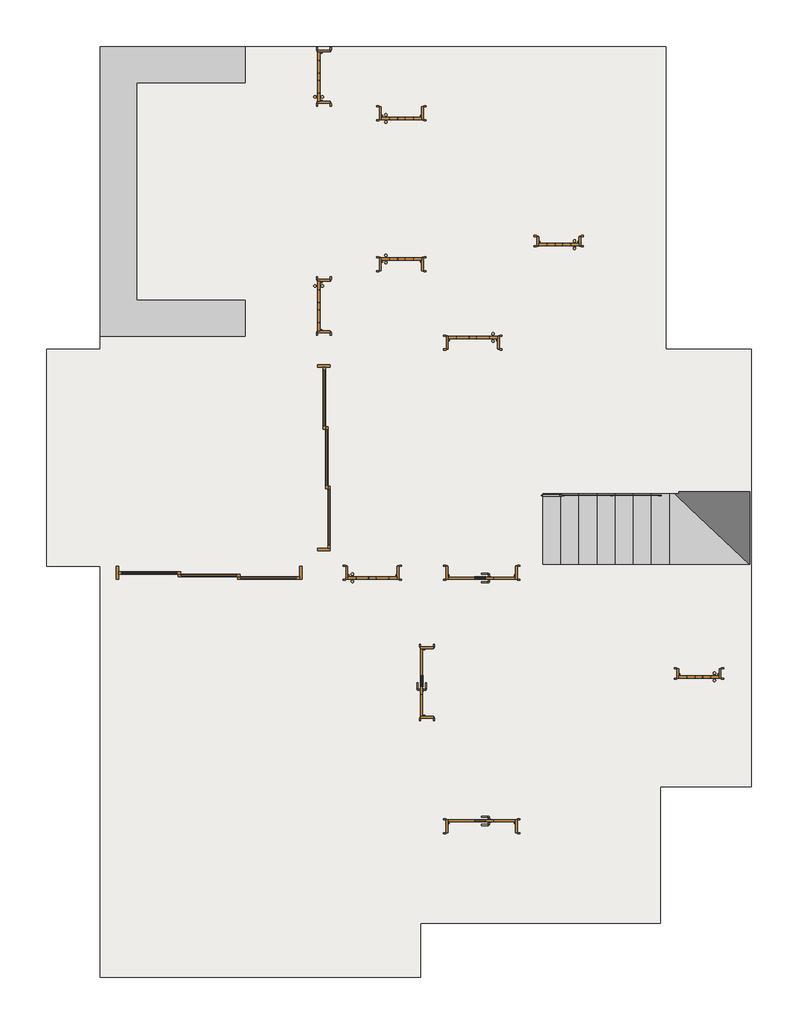
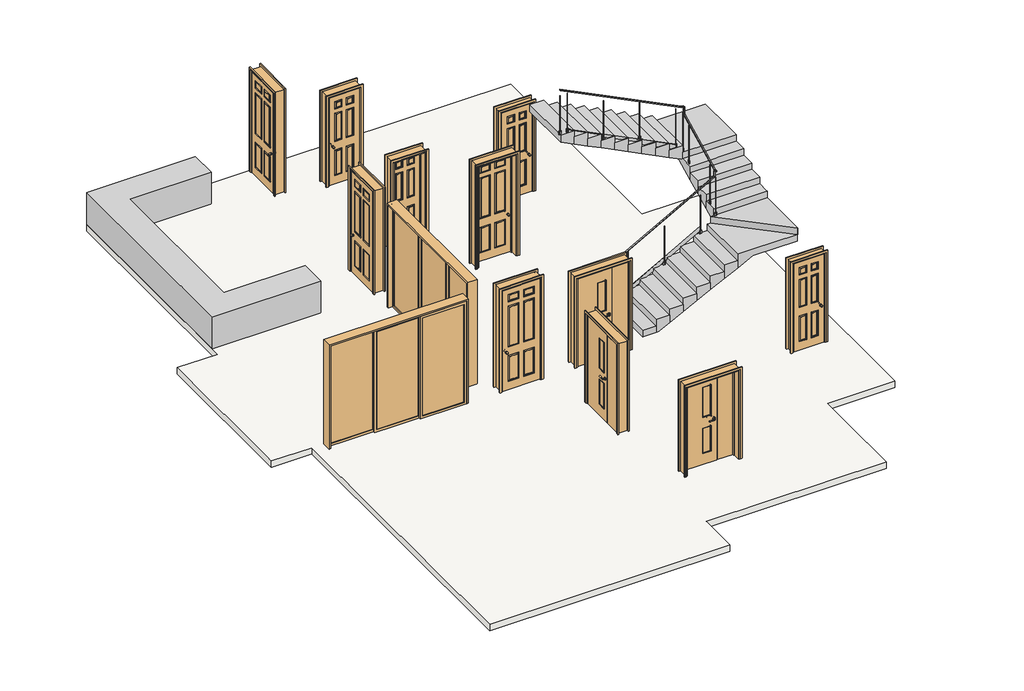
# One storey: 13 doors, 1 furniture element, 1 railing, 1 slab, 1 stair flight.
"""IFC4 building model written with IfcOpenShell, lengths in millimetres."""

from ifc_helpers import new_model, si_unit, frame, origin, place, context, project, spatial, polyline, outline, extrude, faceted_brep, transform, mapped, element, save
from components import d4_91edf99e, d4_bb962316, intays_3_d3_2ab6a75b, intays_3_d3_2b31a8ce, intsgl_9_d1_ce6ece5b, intsgl_9_d1_fdab3a6c, intsgl_9_d2_d60362bb, intsgl_9_d2_d16f3bbe, intsgl_9_d2_8283ee4d, casework_17_casework_17_2f46c277

model = new_model("IFC4")

# Units and contexts
model_context = context("Model", 3, world=origin())
ifc_project = project(units=[si_unit("LENGTHUNIT", "METRE", prefix="MILLI")], contexts=[model_context])

# Site, building, storey
site = spatial("IfcSite", under=ifc_project)
building = spatial("IfcBuilding", under=site)
storey = spatial("IfcBuildingStorey", under=building, Elevation=600.0)

# Doors
placement = place(None, origin())
d4_shape = d4_91edf99e(model_context)
element("IfcDoor", 1, ObjectType="D4", at=placement, inside=storey, context=model_context, shape_type="MappedRepresentation", body=[
    mapped(d4_shape, transform((-10634.1107921, -10590.6567046, 600.0), x_axis=(0.0, 1.0, 0.0), y_axis=(-1.0, 0.0, 0.0), z_axis=(0.0, 0.0, 1.0))),
])
d4_2_shape = d4_bb962316(model_context)
element("IfcDoor", 2, ObjectType="D4", at=placement, inside=storey, context=model_context, shape_type="MappedRepresentation", body=[
    mapped(d4_2_shape, transform((-12453.3527909, -12409.8987034, 600.0), x_axis=(-1.0, 0.0, 0.0), y_axis=(0.0, -1.0, 0.0), z_axis=(0.0, 0.0, 1.0))),
])
intays_3_d3_shape = intays_3_d3_2ab6a75b(model_context)
element("IfcDoor", 3, ObjectType="IntAys (3) : D3", at=placement, inside=storey, context=model_context, shape_type="MappedRepresentation", body=[
    mapped(intays_3_d3_shape, transform((-7780.1107921, -12409.8987034, 600.0), x_axis=(-1.0, 0.0, 0.0), y_axis=(0.0, -1.0, 0.0), z_axis=(0.0, 0.0, 1.0))),
])
element("IfcDoor", 4, ObjectType="IntAys (3) : D3", at=placement, inside=storey, context=model_context, shape_type="MappedRepresentation", body=[
    mapped(intays_3_d3_shape, transform((-8924.1107921, -14468.8987034, 600.0), x_axis=(0.0, 1.0, 0.0), y_axis=(-1.0, 0.0, 0.0), z_axis=(0.0, 0.0, 1.0))),
])
intays_3_d3_2_shape = intays_3_d3_2b31a8ce(model_context)
element("IfcDoor", 5, ObjectType="IntAys (3) : D3", at=placement, inside=storey, context=model_context, shape_type="MappedRepresentation", body=[
    mapped(intays_3_d3_2_shape, transform((-7780.1107921, -16609.8987034, 600.0), x_axis=(-1.0, 0.0, 0.0), y_axis=(0.0, -1.0, 0.0), z_axis=(0.0, 0.0, 1.0))),
])
intsgl_9_d1_shape = intsgl_9_d1_ce6ece5b(model_context)
element("IfcDoor", 6, ObjectType="IntSgl (9) : D1", at=placement, inside=storey, context=model_context, shape_type="MappedRepresentation", body=[
    mapped(intsgl_9_d1_shape, transform((-8164.1107921, -8599.8987034, 600.0), x_axis=(-1.0, 0.0, 0.0), y_axis=(0.0, -1.0, 0.0), z_axis=(0.0, 0.0, 1.0))),
])
element("IfcDoor", 7, ObjectType="IntSgl (9) : D1", at=placement, inside=storey, context=model_context, shape_type="MappedRepresentation", body=[
    mapped(intsgl_9_d1_shape, transform((-10634.1107921, -7994.8987034, 600.0), x_axis=(0.0, -1.0, 0.0), y_axis=(1.0, 0.0, 0.0), z_axis=(0.0, 0.0, 1.0))),
])
element("IfcDoor", 8, ObjectType="IntSgl (9) : D1", at=placement, inside=storey, context=model_context, shape_type="MappedRepresentation", body=[
    mapped(intsgl_9_d1_shape, transform((-9829.1107921, -12409.8987034, 600.0), x_axis=(1.0, 0.0, 0.0), y_axis=(0.0, 1.0, 0.0), z_axis=(0.0, 0.0, 1.0))),
])
intsgl_9_d1_2_shape = intsgl_9_d1_fdab3a6c(model_context)
element("IfcDoor", 9, ObjectType="IntSgl (9) : D1", at=placement, inside=storey, context=model_context, shape_type="MappedRepresentation", body=[
    mapped(intsgl_9_d1_2_shape, transform((-10634.1107921, -4194.8987034, 600.0), x_axis=(0.0, 1.0, 0.0), y_axis=(-1.0, 0.0, 0.0), z_axis=(0.0, 0.0, 1.0))),
])
intsgl_9_d2_shape = intsgl_9_d2_d60362bb(model_context)
element("IfcDoor", 10, ObjectType="IntSgl (9) : D2", at=placement, inside=storey, context=model_context, shape_type="MappedRepresentation", body=[
    mapped(intsgl_9_d2_shape, transform((-9349.1107921, -7299.8987034, 600.0), x_axis=(1.0, 0.0, 0.0), y_axis=(0.0, 1.0, 0.0), z_axis=(0.0, 0.0, 1.0))),
])
intsgl_9_d2_2_shape = intsgl_9_d2_d16f3bbe(model_context)
element("IfcDoor", 11, ObjectType="IntSgl (9) : D2", at=placement, inside=storey, context=model_context, shape_type="MappedRepresentation", body=[
    mapped(intsgl_9_d2_2_shape, transform((-9349.1107921, -4799.8987034, 600.0), x_axis=(1.0, 0.0, 0.0), y_axis=(0.0, 1.0, 0.0), z_axis=(0.0, 0.0, 1.0))),
])
intsgl_9_d2_3_shape = intsgl_9_d2_8283ee4d(model_context)
element("IfcDoor", 12, ObjectType="IntSgl (9) : D2", at=placement, inside=storey, context=model_context, shape_type="MappedRepresentation", body=[
    mapped(intsgl_9_d2_3_shape, transform((-6739.1107921, -6919.8987034, 600.0), x_axis=(-1.0, 0.0, 0.0), y_axis=(0.0, -1.0, 0.0), z_axis=(0.0, 0.0, 1.0))),
])
element("IfcDoor", 13, ObjectType="IntSgl (9) : D2", at=placement, inside=storey, context=model_context, shape_type="MappedRepresentation", body=[
    mapped(intsgl_9_d2_3_shape, transform((-4419.1107921, -14079.8987034, 600.0), x_axis=(-1.0, 0.0, 0.0), y_axis=(0.0, -1.0, 0.0), z_axis=(0.0, 0.0, 1.0))),
])

# Furniture
casework_17_casework_17_shape = casework_17_casework_17_2f46c277(model_context)
element("IfcFurniture", 14, ObjectType="Casework 17 : Casework 17", at=placement, inside=storey, context=model_context, shape_type="MappedRepresentation", body=[
    mapped(casework_17_casework_17_shape, transform((0.0, 0.0, 0.0), x_axis=(1.0, 0.0, 0.0), y_axis=(0.0, 1.0, 0.0), z_axis=(0.0, 0.0, 1.0))),
])

# Railing
element("IfcRailing", 15, at=placement, inside=storey, context=model_context, shape_type="SolidModel", body=[
    faceted_brep([(-7004.1107921, -11120.2987034, 1650.0), (-7004.1107921, -11120.2987034, 1627.1579377), (-7004.1107921, -11140.2987034, 1627.1579377), (-7004.1107921, -11140.2987034, 1650.0), (-7454.1107921, -9889.4987034, 5100.0), (-7454.1107921, -9869.4987034, 5100.0), (-7454.1107921, -9869.4987034, 5077.6393202), (-7454.1107921, -9889.4987034, 5077.6393202), (-4768.7107921, -11120.2987034, 2883.3241379), (-4748.7107921, -11120.2987034, 2871.5165584), (-4748.7107921, -11140.2987034, 2871.5165584), (-4768.7107921, -11140.2987034, 2883.3241379), (-4768.7107921, -11120.2987034, 3007.3), (-4748.7107921, -11120.2987034, 2987.3), (-4748.7107921, -11140.2987034, 2987.3), (-4768.7107921, -11140.2987034, 3007.3), (-4738.7107921, -11120.2987034, 3007.3), (-4738.7107921, -11120.2987034, 2987.3), (-4718.7107921, -11140.2987034, 2987.3), (-4718.7107921, -11140.2987034, 3007.3), (-4738.7107921, -11090.2987034, 3007.3), (-4738.7107921, -11085.5773439, 2987.3), (-4718.7107921, -11085.5773439, 2987.3), (-4718.7107921, -11090.2987034, 3007.3), (-4738.7107921, -9919.4987034, 3592.7), (-4738.7107921, -9899.4987034, 3580.3393202), (-4718.7107921, -9899.4987034, 3580.3393202), (-4718.7107921, -9919.4987034, 3592.7), (-4738.7107921, -9919.4987034, 3757.3), (-4738.7107921, -9899.4987034, 3737.3), (-4718.7107921, -9899.4987034, 3737.3), (-4718.7107921, -9919.4987034, 3757.3), (-4738.7107921, -9889.4987034, 3757.3), (-4738.7107921, -9889.4987034, 3737.3), (-4718.7107921, -9869.4987034, 3737.3), (-4718.7107921, -9869.4987034, 3757.3), (-4768.7107921, -9889.4987034, 3757.3), (-4773.4321517, -9889.4987034, 3737.3), (-4773.4321517, -9869.4987034, 3737.3), (-4768.7107921, -9869.4987034, 3757.3)], [[[0, 1, 2, 3]], [[4, 5, 6, 7]], [[1, 0, 8, 9]], [[2, 1, 9, 10]], [[3, 2, 10, 11]], [[0, 3, 11, 8]], [[9, 8, 12, 13]], [[10, 9, 13, 14]], [[11, 10, 14, 15]], [[8, 11, 15, 12]], [[13, 12, 16, 17]], [[14, 13, 17, 18]], [[15, 14, 18, 19]], [[12, 15, 19, 16]], [[17, 16, 20, 21]], [[18, 17, 21, 22]], [[19, 18, 22, 23]], [[16, 19, 23, 20]], [[21, 20, 24, 25]], [[22, 21, 25, 26]], [[23, 22, 26, 27]], [[20, 23, 27, 24]], [[25, 24, 28, 29]], [[26, 25, 29, 30]], [[27, 26, 30, 31]], [[24, 27, 31, 28]], [[29, 28, 32, 33]], [[30, 29, 33, 34]], [[31, 30, 34, 35]], [[28, 31, 35, 32]], [[33, 32, 36, 37]], [[34, 33, 37, 38]], [[35, 34, 38, 39]], [[32, 35, 39, 36]], [[37, 36, 4, 7]], [[38, 37, 7, 6]], [[39, 38, 6, 5]], [[36, 39, 5, 4]]]),
    extrude(outline(polyline([(-7288.9107921, -9876.9987034), (-7288.9107921, -9881.9987034), (-7293.9107921, -9881.9987034), (-7293.9107921, -9876.9987034), (-7288.9107921, -9876.9987034)])), frame((0.0, 0.0, 4050.0), z_axis=(0.0, 0.0, 1.0), x_axis=(1.0, 0.0, 0.0)), (0.0, 0.0, 1.0), 900.0),
    extrude(outline(polyline([(-7268.9107921, -9881.9987034), (-7268.9107921, -9884.4987034), (-7283.9107921, -9884.4987034), (-7283.9107921, -9881.9987034), (-7268.9107921, -9881.9987034)])), frame((0.0, 0.0, 4050.0), z_axis=(0.0, 0.0, 1.0), x_axis=(1.0, 0.0, 0.0)), (0.0, 0.0, 1.0), 75.0),
    extrude(outline(polyline([(-7268.9107921, -9876.9987034), (-7283.9107921, -9876.9987034), (-7283.9107921, -9874.4987034), (-7268.9107921, -9874.4987034), (-7268.9107921, -9876.9987034)])), frame((0.0, 0.0, 4050.0), z_axis=(0.0, 0.0, 1.0), x_axis=(1.0, 0.0, 0.0)), (0.0, 0.0, 1.0), 75.0),
    extrude(outline(polyline([(-7313.9107921, -9881.9987034), (-7298.9107921, -9881.9987034), (-7298.9107921, -9884.4987034), (-7313.9107921, -9884.4987034), (-7313.9107921, -9881.9987034)])), frame((0.0, 0.0, 4050.0), z_axis=(0.0, 0.0, 1.0), x_axis=(1.0, 0.0, 0.0)), (0.0, 0.0, 1.0), 75.0),
    extrude(outline(polyline([(-7313.9107921, -9876.9987034), (-7313.9107921, -9874.4987034), (-7298.9107921, -9874.4987034), (-7298.9107921, -9876.9987034), (-7313.9107921, -9876.9987034)])), frame((0.0, 0.0, 4050.0), z_axis=(0.0, 0.0, 1.0), x_axis=(1.0, 0.0, 0.0)), (0.0, 0.0, 1.0), 75.0),
    extrude(outline(polyline([(3718.65, -6491.4107921), (4118.65, -7291.4107921), (4100.0, -7291.4107921), (3700.0, -6491.4107921), (3718.65, -6491.4107921)])), frame((0.0, -9886.2235135, 0.0), z_axis=(0.0, 1.0, 0.0), x_axis=(0.0, 0.0, 1.0)), (0.0, 0.0, 1.0), 5.0),
    extrude(outline(polyline([(-6488.9107921, -9876.9987034), (-6488.9107921, -9881.9987034), (-6493.9107921, -9881.9987034), (-6493.9107921, -9876.9987034), (-6488.9107921, -9876.9987034)])), frame((0.0, 0.0, 3600.0), z_axis=(0.0, 0.0, 1.0), x_axis=(1.0, 0.0, 0.0)), (0.0, 0.0, 1.0), 900.0),
    extrude(outline(polyline([(-6468.9107921, -9881.9987034), (-6468.9107921, -9884.4987034), (-6483.9107921, -9884.4987034), (-6483.9107921, -9881.9987034), (-6468.9107921, -9881.9987034)])), frame((0.0, 0.0, 3600.0), z_axis=(0.0, 0.0, 1.0), x_axis=(1.0, 0.0, 0.0)), (0.0, 0.0, 1.0), 75.0),
    extrude(outline(polyline([(-6468.9107921, -9876.9987034), (-6483.9107921, -9876.9987034), (-6483.9107921, -9874.4987034), (-6468.9107921, -9874.4987034), (-6468.9107921, -9876.9987034)])), frame((0.0, 0.0, 3600.0), z_axis=(0.0, 0.0, 1.0), x_axis=(1.0, 0.0, 0.0)), (0.0, 0.0, 1.0), 75.0),
    extrude(outline(polyline([(-6513.9107921, -9881.9987034), (-6498.9107921, -9881.9987034), (-6498.9107921, -9884.4987034), (-6513.9107921, -9884.4987034), (-6513.9107921, -9881.9987034)])), frame((0.0, 0.0, 3600.0), z_axis=(0.0, 0.0, 1.0), x_axis=(1.0, 0.0, 0.0)), (0.0, 0.0, 1.0), 75.0),
    extrude(outline(polyline([(-6513.9107921, -9876.9987034), (-6513.9107921, -9874.4987034), (-6498.9107921, -9874.4987034), (-6498.9107921, -9876.9987034), (-6513.9107921, -9876.9987034)])), frame((0.0, 0.0, 3600.0), z_axis=(0.0, 0.0, 1.0), x_axis=(1.0, 0.0, 0.0)), (0.0, 0.0, 1.0), 75.0),
    extrude(outline(polyline([(3318.65, -5691.4107921), (3718.65, -6491.4107921), (3650.0, -6491.4107921), (3250.0, -5691.4107921), (3318.65, -5691.4107921)])), frame((0.0, -9886.2235135, 0.0), z_axis=(0.0, 1.0, 0.0), x_axis=(0.0, 0.0, 1.0)), (0.0, 0.0, 1.0), 5.0),
    extrude(outline(polyline([(-5688.9107921, -9876.9987034), (-5688.9107921, -9881.9987034), (-5693.9107921, -9881.9987034), (-5693.9107921, -9876.9987034), (-5688.9107921, -9876.9987034)])), frame((0.0, 0.0, 3300.0), z_axis=(0.0, 0.0, 1.0), x_axis=(1.0, 0.0, 0.0)), (0.0, 0.0, 1.0), 900.0),
    extrude(outline(polyline([(-5668.9107921, -9881.9987034), (-5668.9107921, -9884.4987034), (-5683.9107921, -9884.4987034), (-5683.9107921, -9881.9987034), (-5668.9107921, -9881.9987034)])), frame((0.0, 0.0, 3300.0), z_axis=(0.0, 0.0, 1.0), x_axis=(1.0, 0.0, 0.0)), (0.0, 0.0, 1.0), 75.0),
    extrude(outline(polyline([(-5668.9107921, -9876.9987034), (-5683.9107921, -9876.9987034), (-5683.9107921, -9874.4987034), (-5668.9107921, -9874.4987034), (-5668.9107921, -9876.9987034)])), frame((0.0, 0.0, 3300.0), z_axis=(0.0, 0.0, 1.0), x_axis=(1.0, 0.0, 0.0)), (0.0, 0.0, 1.0), 75.0),
    extrude(outline(polyline([(-5713.9107921, -9881.9987034), (-5698.9107921, -9881.9987034), (-5698.9107921, -9884.4987034), (-5713.9107921, -9884.4987034), (-5713.9107921, -9881.9987034)])), frame((0.0, 0.0, 3300.0), z_axis=(0.0, 0.0, 1.0), x_axis=(1.0, 0.0, 0.0)), (0.0, 0.0, 1.0), 75.0),
    extrude(outline(polyline([(-5713.9107921, -9876.9987034), (-5713.9107921, -9874.4987034), (-5698.9107921, -9874.4987034), (-5698.9107921, -9876.9987034), (-5713.9107921, -9876.9987034)])), frame((0.0, 0.0, 3300.0), z_axis=(0.0, 0.0, 1.0), x_axis=(1.0, 0.0, 0.0)), (0.0, 0.0, 1.0), 75.0),
    extrude(outline(polyline([(2918.65, -4891.4107921), (3318.65, -5691.4107921), (3200.0, -5691.4107921), (2800.0, -4891.4107921), (2918.65, -4891.4107921)])), frame((0.0, -9886.2235135, 0.0), z_axis=(0.0, 1.0, 0.0), x_axis=(0.0, 0.0, 1.0)), (0.0, 0.0, 1.0), 5.0),
    extrude(outline(polyline([(-4888.9107921, -9876.9987034), (-4888.9107921, -9881.9987034), (-4893.9107921, -9881.9987034), (-4893.9107921, -9876.9987034), (-4888.9107921, -9876.9987034)])), frame((0.0, 0.0, 2850.0), z_axis=(0.0, 0.0, 1.0), x_axis=(1.0, 0.0, 0.0)), (0.0, 0.0, 1.0), 900.0),
    extrude(outline(polyline([(-4868.9107921, -9881.9987034), (-4868.9107921, -9884.4987034), (-4883.9107921, -9884.4987034), (-4883.9107921, -9881.9987034), (-4868.9107921, -9881.9987034)])), frame((0.0, 0.0, 2850.0), z_axis=(0.0, 0.0, 1.0), x_axis=(1.0, 0.0, 0.0)), (0.0, 0.0, 1.0), 75.0),
    extrude(outline(polyline([(-4868.9107921, -9876.9987034), (-4883.9107921, -9876.9987034), (-4883.9107921, -9874.4987034), (-4868.9107921, -9874.4987034), (-4868.9107921, -9876.9987034)])), frame((0.0, 0.0, 2850.0), z_axis=(0.0, 0.0, 1.0), x_axis=(1.0, 0.0, 0.0)), (0.0, 0.0, 1.0), 75.0),
    extrude(outline(polyline([(-4913.9107921, -9881.9987034), (-4898.9107921, -9881.9987034), (-4898.9107921, -9884.4987034), (-4913.9107921, -9884.4987034), (-4913.9107921, -9881.9987034)])), frame((0.0, 0.0, 2850.0), z_axis=(0.0, 0.0, 1.0), x_axis=(1.0, 0.0, 0.0)), (0.0, 0.0, 1.0), 75.0),
    extrude(outline(polyline([(-4913.9107921, -9876.9987034), (-4913.9107921, -9874.4987034), (-4898.9107921, -9874.4987034), (-4898.9107921, -9876.9987034), (-4913.9107921, -9876.9987034)])), frame((0.0, 0.0, 2850.0), z_axis=(0.0, 0.0, 1.0), x_axis=(1.0, 0.0, 0.0)), (0.0, 0.0, 1.0), 75.0),
    extrude(outline(polyline([(-4726.2107921, -10107.3987034), (-4731.2107921, -10107.3987034), (-4731.2107921, -10102.3987034), (-4726.2107921, -10102.3987034), (-4726.2107921, -10107.3987034)])), frame((0.0, 0.0, 2550.0), z_axis=(0.0, 0.0, 1.0), x_axis=(1.0, 0.0, 0.0)), (0.0, 0.0, 1.0), 900.0),
    extrude(outline(polyline([(-4731.2107921, -10127.3987034), (-4733.7107921, -10127.3987034), (-4733.7107921, -10112.3987034), (-4731.2107921, -10112.3987034), (-4731.2107921, -10127.3987034)])), frame((0.0, 0.0, 2550.0), z_axis=(0.0, 0.0, 1.0), x_axis=(1.0, 0.0, 0.0)), (0.0, 0.0, 1.0), 75.0),
    extrude(outline(polyline([(-4726.2107921, -10127.3987034), (-4726.2107921, -10112.3987034), (-4723.7107921, -10112.3987034), (-4723.7107921, -10127.3987034), (-4726.2107921, -10127.3987034)])), frame((0.0, 0.0, 2550.0), z_axis=(0.0, 0.0, 1.0), x_axis=(1.0, 0.0, 0.0)), (0.0, 0.0, 1.0), 75.0),
    extrude(outline(polyline([(-4731.2107921, -10082.3987034), (-4731.2107921, -10097.3987034), (-4733.7107921, -10097.3987034), (-4733.7107921, -10082.3987034), (-4731.2107921, -10082.3987034)])), frame((0.0, 0.0, 2550.0), z_axis=(0.0, 0.0, 1.0), x_axis=(1.0, 0.0, 0.0)), (0.0, 0.0, 1.0), 75.0),
    extrude(outline(polyline([(-4726.2107921, -10082.3987034), (-4723.7107921, -10082.3987034), (-4723.7107921, -10097.3987034), (-4726.2107921, -10097.3987034), (-4726.2107921, -10082.3987034)])), frame((0.0, 0.0, 2550.0), z_axis=(0.0, 0.0, 1.0), x_axis=(1.0, 0.0, 0.0)), (0.0, 0.0, 1.0), 75.0),
    extrude(outline(polyline([(-4726.2107921, -10907.3987034), (-4731.2107921, -10907.3987034), (-4731.2107921, -10902.3987034), (-4726.2107921, -10902.3987034), (-4726.2107921, -10907.3987034)])), frame((0.0, 0.0, 2100.0), z_axis=(0.0, 0.0, 1.0), x_axis=(1.0, 0.0, 0.0)), (0.0, 0.0, 1.0), 900.0),
    extrude(outline(polyline([(-4731.2107921, -10927.3987034), (-4733.7107921, -10927.3987034), (-4733.7107921, -10912.3987034), (-4731.2107921, -10912.3987034), (-4731.2107921, -10927.3987034)])), frame((0.0, 0.0, 2100.0), z_axis=(0.0, 0.0, 1.0), x_axis=(1.0, 0.0, 0.0)), (0.0, 0.0, 1.0), 75.0),
    extrude(outline(polyline([(-4726.2107921, -10927.3987034), (-4726.2107921, -10912.3987034), (-4723.7107921, -10912.3987034), (-4723.7107921, -10927.3987034), (-4726.2107921, -10927.3987034)])), frame((0.0, 0.0, 2100.0), z_axis=(0.0, 0.0, 1.0), x_axis=(1.0, 0.0, 0.0)), (0.0, 0.0, 1.0), 75.0),
    extrude(outline(polyline([(-4731.2107921, -10882.3987034), (-4731.2107921, -10897.3987034), (-4733.7107921, -10897.3987034), (-4733.7107921, -10882.3987034), (-4731.2107921, -10882.3987034)])), frame((0.0, 0.0, 2100.0), z_axis=(0.0, 0.0, 1.0), x_axis=(1.0, 0.0, 0.0)), (0.0, 0.0, 1.0), 75.0),
    extrude(outline(polyline([(-4726.2107921, -10882.3987034), (-4723.7107921, -10882.3987034), (-4723.7107921, -10897.3987034), (-4726.2107921, -10897.3987034), (-4726.2107921, -10882.3987034)])), frame((0.0, 0.0, 2100.0), z_axis=(0.0, 0.0, 1.0), x_axis=(1.0, 0.0, 0.0)), (0.0, 0.0, 1.0), 75.0),
    extrude(outline(polyline([(-5068.9107921, -11132.7987034), (-5068.9107921, -11127.7987034), (-5063.9107921, -11127.7987034), (-5063.9107921, -11132.7987034), (-5068.9107921, -11132.7987034)])), frame((0.0, 0.0, 1650.0), z_axis=(0.0, 0.0, 1.0), x_axis=(1.0, 0.0, 0.0)), (0.0, 0.0, 1.0), 900.0),
    extrude(outline(polyline([(-5088.9107921, -11127.7987034), (-5088.9107921, -11125.2987034), (-5073.9107921, -11125.2987034), (-5073.9107921, -11127.7987034), (-5088.9107921, -11127.7987034)])), frame((0.0, 0.0, 1650.0), z_axis=(0.0, 0.0, 1.0), x_axis=(1.0, 0.0, 0.0)), (0.0, 0.0, 1.0), 75.0),
    extrude(outline(polyline([(-5088.9107921, -11132.7987034), (-5073.9107921, -11132.7987034), (-5073.9107921, -11135.2987034), (-5088.9107921, -11135.2987034), (-5088.9107921, -11132.7987034)])), frame((0.0, 0.0, 1650.0), z_axis=(0.0, 0.0, 1.0), x_axis=(1.0, 0.0, 0.0)), (0.0, 0.0, 1.0), 75.0),
    extrude(outline(polyline([(-5043.9107921, -11127.7987034), (-5058.9107921, -11127.7987034), (-5058.9107921, -11125.2987034), (-5043.9107921, -11125.2987034), (-5043.9107921, -11127.7987034)])), frame((0.0, 0.0, 1650.0), z_axis=(0.0, 0.0, 1.0), x_axis=(1.0, 0.0, 0.0)), (0.0, 0.0, 1.0), 75.0),
    extrude(outline(polyline([(-5043.9107921, -11132.7987034), (-5043.9107921, -11135.2987034), (-5058.9107921, -11135.2987034), (-5058.9107921, -11132.7987034), (-5043.9107921, -11132.7987034)])), frame((0.0, 0.0, 1650.0), z_axis=(0.0, 0.0, 1.0), x_axis=(1.0, 0.0, 0.0)), (0.0, 0.0, 1.0), 75.0),
    extrude(outline(polyline([(1377.6965517, -5866.4107921), (1279.3103448, -5866.4107921), (1720.6896552, -5066.4107921), (1819.0758621, -5066.4107921), (1377.6965517, -5866.4107921)])), frame((0.0, -11128.5738933, 0.0), z_axis=(0.0, 1.0, 0.0), x_axis=(0.0, 0.0, 1.0)), (0.0, 0.0, 1.0), 5.0),
    extrude(outline(polyline([(-5868.9107921, -11132.7987034), (-5868.9107921, -11127.7987034), (-5863.9107921, -11127.7987034), (-5863.9107921, -11132.7987034), (-5868.9107921, -11132.7987034)])), frame((0.0, 0.0, 1200.0), z_axis=(0.0, 0.0, 1.0), x_axis=(1.0, 0.0, 0.0)), (0.0, 0.0, 1.0), 900.0),
    extrude(outline(polyline([(-5888.9107921, -11127.7987034), (-5888.9107921, -11125.2987034), (-5873.9107921, -11125.2987034), (-5873.9107921, -11127.7987034), (-5888.9107921, -11127.7987034)])), frame((0.0, 0.0, 1200.0), z_axis=(0.0, 0.0, 1.0), x_axis=(1.0, 0.0, 0.0)), (0.0, 0.0, 1.0), 75.0),
    extrude(outline(polyline([(-5888.9107921, -11132.7987034), (-5873.9107921, -11132.7987034), (-5873.9107921, -11135.2987034), (-5888.9107921, -11135.2987034), (-5888.9107921, -11132.7987034)])), frame((0.0, 0.0, 1200.0), z_axis=(0.0, 0.0, 1.0), x_axis=(1.0, 0.0, 0.0)), (0.0, 0.0, 1.0), 75.0),
    extrude(outline(polyline([(-5843.9107921, -11127.7987034), (-5858.9107921, -11127.7987034), (-5858.9107921, -11125.2987034), (-5843.9107921, -11125.2987034), (-5843.9107921, -11127.7987034)])), frame((0.0, 0.0, 1200.0), z_axis=(0.0, 0.0, 1.0), x_axis=(1.0, 0.0, 0.0)), (0.0, 0.0, 1.0), 75.0),
    extrude(outline(polyline([(-5843.9107921, -11132.7987034), (-5843.9107921, -11135.2987034), (-5858.9107921, -11135.2987034), (-5858.9107921, -11132.7987034), (-5843.9107921, -11132.7987034)])), frame((0.0, 0.0, 1200.0), z_axis=(0.0, 0.0, 1.0), x_axis=(1.0, 0.0, 0.0)), (0.0, 0.0, 1.0), 75.0),
    extrude(outline(polyline([(936.3172414, -6666.4107921), (829.3103448, -6666.4107921), (1270.6896552, -5866.4107921), (1377.6965517, -5866.4107921), (936.3172414, -6666.4107921)])), frame((0.0, -11128.5738933, 0.0), z_axis=(0.0, 1.0, 0.0), x_axis=(0.0, 0.0, 1.0)), (0.0, 0.0, 1.0), 5.0),
    extrude(outline(polyline([(-6668.9107921, -11132.7987034), (-6668.9107921, -11127.7987034), (-6663.9107921, -11127.7987034), (-6663.9107921, -11132.7987034), (-6668.9107921, -11132.7987034)])), frame((0.0, 0.0, 900.0), z_axis=(0.0, 0.0, 1.0), x_axis=(1.0, 0.0, 0.0)), (0.0, 0.0, 1.0), 900.0),
    extrude(outline(polyline([(-6688.9107921, -11127.7987034), (-6688.9107921, -11125.2987034), (-6673.9107921, -11125.2987034), (-6673.9107921, -11127.7987034), (-6688.9107921, -11127.7987034)])), frame((0.0, 0.0, 900.0), z_axis=(0.0, 0.0, 1.0), x_axis=(1.0, 0.0, 0.0)), (0.0, 0.0, 1.0), 75.0),
    extrude(outline(polyline([(-6688.9107921, -11132.7987034), (-6673.9107921, -11132.7987034), (-6673.9107921, -11135.2987034), (-6688.9107921, -11135.2987034), (-6688.9107921, -11132.7987034)])), frame((0.0, 0.0, 900.0), z_axis=(0.0, 0.0, 1.0), x_axis=(1.0, 0.0, 0.0)), (0.0, 0.0, 1.0), 75.0),
    extrude(outline(polyline([(-6643.9107921, -11127.7987034), (-6658.9107921, -11127.7987034), (-6658.9107921, -11125.2987034), (-6643.9107921, -11125.2987034), (-6643.9107921, -11127.7987034)])), frame((0.0, 0.0, 900.0), z_axis=(0.0, 0.0, 1.0), x_axis=(1.0, 0.0, 0.0)), (0.0, 0.0, 1.0), 75.0),
    extrude(outline(polyline([(-6643.9107921, -11132.7987034), (-6643.9107921, -11135.2987034), (-6658.9107921, -11135.2987034), (-6658.9107921, -11132.7987034), (-6643.9107921, -11132.7987034)])), frame((0.0, 0.0, 900.0), z_axis=(0.0, 0.0, 1.0), x_axis=(1.0, 0.0, 0.0)), (0.0, 0.0, 1.0), 75.0),
    extrude(outline(polyline([(-4726.2107921, -9881.9987034), (-4731.2107921, -9881.9987034), (-4731.2107921, -9876.9987034), (-4726.2107921, -9876.9987034), (-4726.2107921, -9881.9987034)])), frame((0.0, 0.0, 2700.0), z_axis=(0.0, 0.0, 1.0), x_axis=(1.0, 0.0, 0.0)), (0.0, 0.0, 1.0), 900.0),
    extrude(outline(polyline([(-4731.2107921, -9901.9987034), (-4733.7107921, -9901.9987034), (-4733.7107921, -9886.9987034), (-4731.2107921, -9886.9987034), (-4731.2107921, -9901.9987034)])), frame((0.0, 0.0, 2700.0), z_axis=(0.0, 0.0, 1.0), x_axis=(1.0, 0.0, 0.0)), (0.0, 0.0, 1.0), 75.0),
    extrude(outline(polyline([(-4726.2107921, -9901.9987034), (-4726.2107921, -9886.9987034), (-4723.7107921, -9886.9987034), (-4723.7107921, -9901.9987034), (-4726.2107921, -9901.9987034)])), frame((0.0, 0.0, 2700.0), z_axis=(0.0, 0.0, 1.0), x_axis=(1.0, 0.0, 0.0)), (0.0, 0.0, 1.0), 75.0),
    extrude(outline(polyline([(-4731.2107921, -9856.9987034), (-4731.2107921, -9871.9987034), (-4733.7107921, -9871.9987034), (-4733.7107921, -9856.9987034), (-4731.2107921, -9856.9987034)])), frame((0.0, 0.0, 2700.0), z_axis=(0.0, 0.0, 1.0), x_axis=(1.0, 0.0, 0.0)), (0.0, 0.0, 1.0), 75.0),
    extrude(outline(polyline([(-4726.2107921, -9856.9987034), (-4723.7107921, -9856.9987034), (-4723.7107921, -9871.9987034), (-4726.2107921, -9871.9987034), (-4726.2107921, -9856.9987034)])), frame((0.0, 0.0, 2700.0), z_axis=(0.0, 0.0, 1.0), x_axis=(1.0, 0.0, 0.0)), (0.0, 0.0, 1.0), 75.0),
    extrude(outline(polyline([(-4731.2107921, -11132.7987034), (-4731.2107921, -11127.7987034), (-4726.2107921, -11127.7987034), (-4726.2107921, -11132.7987034), (-4731.2107921, -11132.7987034)])), frame((0.0, 0.0, 1950.0), z_axis=(0.0, 0.0, 1.0), x_axis=(1.0, 0.0, 0.0)), (0.0, 0.0, 1.0), 900.0),
    extrude(outline(polyline([(-4751.2107921, -11127.7987034), (-4751.2107921, -11125.2987034), (-4736.2107921, -11125.2987034), (-4736.2107921, -11127.7987034), (-4751.2107921, -11127.7987034)])), frame((0.0, 0.0, 1950.0), z_axis=(0.0, 0.0, 1.0), x_axis=(1.0, 0.0, 0.0)), (0.0, 0.0, 1.0), 75.0),
    extrude(outline(polyline([(-4751.2107921, -11132.7987034), (-4736.2107921, -11132.7987034), (-4736.2107921, -11135.2987034), (-4751.2107921, -11135.2987034), (-4751.2107921, -11132.7987034)])), frame((0.0, 0.0, 1950.0), z_axis=(0.0, 0.0, 1.0), x_axis=(1.0, 0.0, 0.0)), (0.0, 0.0, 1.0), 75.0),
    extrude(outline(polyline([(-4706.2107921, -11127.7987034), (-4721.2107921, -11127.7987034), (-4721.2107921, -11125.2987034), (-4706.2107921, -11125.2987034), (-4706.2107921, -11127.7987034)])), frame((0.0, 0.0, 1950.0), z_axis=(0.0, 0.0, 1.0), x_axis=(1.0, 0.0, 0.0)), (0.0, 0.0, 1.0), 75.0),
    extrude(outline(polyline([(-4706.2107921, -11132.7987034), (-4706.2107921, -11135.2987034), (-4721.2107921, -11135.2987034), (-4721.2107921, -11132.7987034), (-4706.2107921, -11132.7987034)])), frame((0.0, 0.0, 1950.0), z_axis=(0.0, 0.0, 1.0), x_axis=(1.0, 0.0, 0.0)), (0.0, 0.0, 1.0), 75.0),
    extrude(outline(polyline([(-7449.6107921, -9876.9987034), (-7449.6107921, -9881.9987034), (-7454.6107921, -9881.9987034), (-7454.6107921, -9876.9987034), (-7449.6107921, -9876.9987034)])), frame((0.0, 0.0, 4050.0), z_axis=(0.0, 0.0, 1.0), x_axis=(1.0, 0.0, 0.0)), (0.0, 0.0, 1.0), 900.0),
    extrude(outline(polyline([(-7429.6107921, -9881.9987034), (-7429.6107921, -9884.4987034), (-7444.6107921, -9884.4987034), (-7444.6107921, -9881.9987034), (-7429.6107921, -9881.9987034)])), frame((0.0, 0.0, 4050.0), z_axis=(0.0, 0.0, 1.0), x_axis=(1.0, 0.0, 0.0)), (0.0, 0.0, 1.0), 75.0),
    extrude(outline(polyline([(-7429.6107921, -9876.9987034), (-7444.6107921, -9876.9987034), (-7444.6107921, -9874.4987034), (-7429.6107921, -9874.4987034), (-7429.6107921, -9876.9987034)])), frame((0.0, 0.0, 4050.0), z_axis=(0.0, 0.0, 1.0), x_axis=(1.0, 0.0, 0.0)), (0.0, 0.0, 1.0), 75.0),
    extrude(outline(polyline([(-7474.6107921, -9881.9987034), (-7459.6107921, -9881.9987034), (-7459.6107921, -9884.4987034), (-7474.6107921, -9884.4987034), (-7474.6107921, -9881.9987034)])), frame((0.0, 0.0, 4050.0), z_axis=(0.0, 0.0, 1.0), x_axis=(1.0, 0.0, 0.0)), (0.0, 0.0, 1.0), 75.0),
    extrude(outline(polyline([(-7474.6107921, -9876.9987034), (-7474.6107921, -9874.4987034), (-7459.6107921, -9874.4987034), (-7459.6107921, -9876.9987034), (-7474.6107921, -9876.9987034)])), frame((0.0, 0.0, 4050.0), z_axis=(0.0, 0.0, 1.0), x_axis=(1.0, 0.0, 0.0)), (0.0, 0.0, 1.0), 75.0),
    extrude(outline(polyline([(-7004.6107921, -11132.7987034), (-7004.6107921, -11127.7987034), (-6999.6107921, -11127.7987034), (-6999.6107921, -11132.7987034), (-7004.6107921, -11132.7987034)])), frame((0.0, 0.0, 750.0), z_axis=(0.0, 0.0, 1.0), x_axis=(1.0, 0.0, 0.0)), (0.0, 0.0, 1.0), 900.0),
    extrude(outline(polyline([(-7024.6107921, -11127.7987034), (-7024.6107921, -11125.2987034), (-7009.6107921, -11125.2987034), (-7009.6107921, -11127.7987034), (-7024.6107921, -11127.7987034)])), frame((0.0, 0.0, 750.0), z_axis=(0.0, 0.0, 1.0), x_axis=(1.0, 0.0, 0.0)), (0.0, 0.0, 1.0), 75.0),
    extrude(outline(polyline([(-7024.6107921, -11132.7987034), (-7009.6107921, -11132.7987034), (-7009.6107921, -11135.2987034), (-7024.6107921, -11135.2987034), (-7024.6107921, -11132.7987034)])), frame((0.0, 0.0, 750.0), z_axis=(0.0, 0.0, 1.0), x_axis=(1.0, 0.0, 0.0)), (0.0, 0.0, 1.0), 75.0),
    extrude(outline(polyline([(-6979.6107921, -11127.7987034), (-6994.6107921, -11127.7987034), (-6994.6107921, -11125.2987034), (-6979.6107921, -11125.2987034), (-6979.6107921, -11127.7987034)])), frame((0.0, 0.0, 750.0), z_axis=(0.0, 0.0, 1.0), x_axis=(1.0, 0.0, 0.0)), (0.0, 0.0, 1.0), 75.0),
    extrude(outline(polyline([(-6979.6107921, -11132.7987034), (-6979.6107921, -11135.2987034), (-6994.6107921, -11135.2987034), (-6994.6107921, -11132.7987034), (-6979.6107921, -11132.7987034)])), frame((0.0, 0.0, 750.0), z_axis=(0.0, 0.0, 1.0), x_axis=(1.0, 0.0, 0.0)), (0.0, 0.0, 1.0), 75.0),
])

# Slab
element("IfcSlab", 16, ObjectType="01-FLOOR MAIN", at=placement, inside=storey, context=model_context, shape_type="SweptSolid", body=[
    extrude(outline(polyline([(-9988.4991549, -3694.8987034), (-4964.1107921, -3694.8987034), (-4964.1107921, -8704.8987034), (-3554.1107921, -8704.8987034), (-3554.1107921, -15954.8987034), (-5054.1107921, -15954.8987034), (-5054.1107921, -16714.8987034), (-5054.1107921, -18214.8987034), (-9029.1107921, -18214.8987034), (-9029.1107921, -19114.8987034), (-14339.1107921, -19114.8987034), (-14339.1107921, -12304.8987034), (-15231.6107921, -12304.8987034), (-15231.6107921, -8704.8987034), (-14339.1107921, -8704.8987034), (-14339.1107921, -3694.8987034), (-9988.4991549, -3694.8987034)])), frame((0.0, 0.0, 450.0), z_axis=(0.0, 0.0, 1.0), x_axis=(1.0, 0.0, 0.0)), (0.0, 0.0, 1.0), 150.0),
])

# Stair flight
element("IfcStairFlight", 17, ObjectType="M_Monolithic Run", at=placement, inside=storey, context=model_context, shape_type="Brep", body=[
    faceted_brep([(-6704.1107921, -11104.8987034, 750.0), (-7004.1107921, -11104.8987034, 750.0), (-7004.1107921, -12269.8987034, 750.0), (-6704.1107921, -12269.8987034, 750.0), (-6704.1107921, -11104.8987034, 600.0), (-7004.1107921, -11104.8987034, 600.0), (-7004.1107921, -12269.8987034, 600.0), (-6704.1107921, -12269.8987034, 600.0), (-6404.1107921, -11104.8987034, 900.0), (-6704.1107921, -11104.8987034, 900.0), (-6704.1107921, -12269.8987034, 900.0), (-6404.1107921, -12269.8987034, 900.0), (-6404.1107921, -11104.8987034, 732.2949017), (-6668.7005955, -11104.8987034, 600.0), (-6668.7005955, -12269.8987034, 600.0), (-6404.1107921, -12269.8987034, 732.2949017), (-6104.1107921, -11104.8987034, 1050.0), (-6404.1107921, -11104.8987034, 1050.0), (-6404.1107921, -12269.8987034, 1050.0), (-6104.1107921, -12269.8987034, 1050.0), (-6104.1107921, -11104.8987034, 882.2949017), (-6104.1107921, -12269.8987034, 882.2949017), (-5804.1107921, -11104.8987034, 1200.0), (-6104.1107921, -11104.8987034, 1200.0), (-6104.1107921, -12269.8987034, 1200.0), (-5804.1107921, -12269.8987034, 1200.0), (-5804.1107921, -11104.8987034, 1032.2949017), (-5804.1107921, -12269.8987034, 1032.2949017), (-5504.1107921, -11104.8987034, 1350.0), (-5804.1107921, -11104.8987034, 1350.0), (-5804.1107921, -12269.8987034, 1350.0), (-5504.1107921, -12269.8987034, 1350.0), (-5504.1107921, -11104.8987034, 1182.2949017), (-5504.1107921, -12269.8987034, 1182.2949017), (-5204.1107921, -11104.8987034, 1500.0), (-5504.1107921, -11104.8987034, 1500.0), (-5504.1107921, -12269.8987034, 1500.0), (-5204.1107921, -12269.8987034, 1500.0), (-5204.1107921, -11104.8987034, 1332.2949017), (-5204.1107921, -12269.8987034, 1332.2949017), (-4904.1107921, -11104.8987034, 1650.0), (-5204.1107921, -11104.8987034, 1650.0), (-5204.1107921, -12269.8987034, 1650.0), (-4904.1107921, -12269.8987034, 1650.0), (-4904.1107921, -11104.8987034, 1482.2949017), (-4904.1107921, -12269.8987034, 1482.2949017), (-4829.1107921, -11104.8987034, 1800.0), (-4904.1107921, -11104.8987034, 1800.0), (-4904.1107921, -12269.8987034, 1800.0), (-4568.7005955, -12269.8987034, 1800.0), (-3591.2982921, -12269.8987034, 1800.0), (-4568.7005955, -11349.9906532, 1800.0), (-4829.1107921, -11104.8987034, 1519.7949017), (-4568.7005955, -12269.8987034, 1650.0), (-3591.2982921, -12269.8987034, 1650.0), (-4754.1107921, -11104.8987034, 1950.0), (-4829.1107921, -11104.8987034, 1950.0), (-3591.2982921, -12269.8987034, 1950.0), (-3574.1107921, -12269.8987034, 1950.0), (-3574.1107921, -11104.8987034, 1950.0), (-4754.1107921, -11104.8987034, 1800.0), (-4568.7005955, -11104.8987034, 1800.0), (-4568.7005955, -11104.8987034, 1650.0), (-3574.1107921, -12269.8987034, 1800.0), (-4754.1107921, -11104.8987034, 2100.0), (-3574.1107921, -11104.8987034, 2100.0), (-3574.1107921, -11069.4885068, 2100.0), (-3574.1107921, -10804.8987034, 2100.0), (-4754.1107921, -10804.8987034, 2100.0), (-4754.1107921, -11069.4885068, 2100.0), (-4754.1107921, -10804.8987034, 1932.2949017), (-4754.1107921, -11069.4885068, 1800.0), (-3574.1107921, -11104.8987034, 1800.0), (-3574.1107921, -11069.4885068, 1800.0), (-3574.1107921, -10804.8987034, 1932.2949017), (-4754.1107921, -10504.8987034, 2250.0), (-4754.1107921, -10804.8987034, 2250.0), (-3574.1107921, -10804.8987034, 2250.0), (-3574.1107921, -10504.8987034, 2250.0), (-4754.1107921, -10504.8987034, 2082.2949017), (-3574.1107921, -10504.8987034, 2082.2949017), (-4754.1107921, -10204.8987034, 2400.0), (-4754.1107921, -10504.8987034, 2400.0), (-3574.1107921, -10504.8987034, 2400.0), (-3574.1107921, -10204.8987034, 2400.0), (-4754.1107921, -10204.8987034, 2232.2949017), (-3574.1107921, -10204.8987034, 2232.2949017), (-4754.1107921, -9904.8987034, 2550.0), (-4754.1107921, -10204.8987034, 2550.0), (-3574.1107921, -10204.8987034, 2550.0), (-3574.1107921, -9904.8987034, 2550.0), (-4754.1107921, -9569.4885068, 2550.0), (-3574.1107921, -9904.8987034, 2382.2949017), (-4754.1107921, -9904.8987034, 2700.0), (-3574.1107921, -9904.8987034, 2700.0), (-3574.1107921, -9569.4885068, 2700.0), (-3574.1107921, -8734.8987034, 2700.0), (-4754.1107921, -8734.8987034, 2700.0), (-3574.1107921, -9569.4885068, 2550.0), (-3574.1107921, -8734.8987034, 2550.0), (-4754.1107921, -8734.8987034, 2550.0), (-4754.1107921, -9904.8987034, 2850.0), (-4754.1107921, -8734.8987034, 2850.0), (-4789.5209887, -8734.8987034, 2850.0), (-5054.1107921, -8734.8987034, 2850.0), (-5054.1107921, -9904.8987034, 2850.0), (-4789.5209887, -9904.8987034, 2850.0), (-5054.1107921, -9904.8987034, 2682.2949017), (-4789.5209887, -9904.8987034, 2550.0), (-4789.5209887, -8734.8987034, 2550.0), (-5054.1107921, -8734.8987034, 2682.2949017), (-5354.1107921, -9904.8987034, 3000.0), (-5054.1107921, -9904.8987034, 3000.0), (-5054.1107921, -8734.8987034, 3000.0), (-5354.1107921, -8734.8987034, 3000.0), (-5354.1107921, -9904.8987034, 2832.2949017), (-5354.1107921, -8734.8987034, 2832.2949017), (-5654.1107921, -9904.8987034, 3150.0), (-5354.1107921, -9904.8987034, 3150.0), (-5354.1107921, -8734.8987034, 3150.0), (-5654.1107921, -8734.8987034, 3150.0), (-5654.1107921, -9904.8987034, 2982.2949017), (-5654.1107921, -8734.8987034, 2982.2949017), (-5954.1107921, -9904.8987034, 3300.0), (-5654.1107921, -9904.8987034, 3300.0), (-5654.1107921, -8734.8987034, 3300.0), (-5954.1107921, -8734.8987034, 3300.0), (-5954.1107921, -9904.8987034, 3132.2949017), (-5954.1107921, -8734.8987034, 3132.2949017), (-6254.1107921, -9904.8987034, 3450.0), (-5954.1107921, -9904.8987034, 3450.0), (-5954.1107921, -8734.8987034, 3450.0), (-6254.1107921, -8734.8987034, 3450.0), (-6254.1107921, -9904.8987034, 3282.2949017), (-6254.1107921, -8734.8987034, 3282.2949017), (-6554.1107921, -9904.8987034, 3600.0), (-6254.1107921, -9904.8987034, 3600.0), (-6254.1107921, -8734.8987034, 3600.0), (-6554.1107921, -8734.8987034, 3600.0), (-6554.1107921, -9904.8987034, 3432.2949017), (-6554.1107921, -8734.8987034, 3432.2949017), (-6854.1107921, -9904.8987034, 3750.0), (-6554.1107921, -9904.8987034, 3750.0), (-6554.1107921, -8734.8987034, 3750.0), (-6854.1107921, -8734.8987034, 3750.0), (-6854.1107921, -9904.8987034, 3582.2949017), (-6854.1107921, -8734.8987034, 3582.2949017), (-7154.1107921, -9904.8987034, 3900.0), (-6854.1107921, -9904.8987034, 3900.0), (-6854.1107921, -8734.8987034, 3900.0), (-7154.1107921, -8734.8987034, 3900.0), (-7154.1107921, -9904.8987034, 3732.2949017), (-7154.1107921, -8734.8987034, 3732.2949017), (-7454.1107921, -9904.8987034, 4050.0), (-7154.1107921, -9904.8987034, 4050.0), (-7154.1107921, -8734.8987034, 4050.0), (-7454.1107921, -8734.8987034, 4050.0), (-7454.1107921, -9904.8987034, 3882.2949017), (-7454.1107921, -8734.8987034, 3882.2949017), (-4568.7005955, -11349.9906532, 1650.0), (-4568.7005955, -11349.9906532, 1800.0)], [[[0, 1, 2, 3]], [[1, 0, 4, 5]], [[2, 1, 5, 6]], [[3, 2, 6, 7]], [[8, 9, 10, 11]], [[4, 0, 9, 8, 12, 13]], [[0, 3, 10, 9]], [[3, 7, 14, 15, 11, 10]], [[16, 17, 18, 19]], [[17, 16, 20, 12, 8]], [[8, 11, 18, 17]], [[19, 18, 11, 15, 21]], [[22, 23, 24, 25]], [[23, 22, 26, 20, 16]], [[16, 19, 24, 23]], [[25, 24, 19, 21, 27]], [[28, 29, 30, 31]], [[29, 28, 32, 26, 22]], [[22, 25, 30, 29]], [[31, 30, 25, 27, 33]], [[34, 35, 36, 37]], [[35, 34, 38, 32, 28]], [[28, 31, 36, 35]], [[37, 36, 31, 33, 39]], [[40, 41, 42, 43]], [[41, 40, 44, 38, 34]], [[34, 37, 42, 41]], [[43, 42, 37, 39, 45]], [[46, 47, 48, 49, 50, 51]], [[47, 46, 52, 44, 40]], [[40, 43, 48, 47]], [[48, 43, 45, 53, 54, 50, 49]], [[55, 56, 57, 58, 59]], [[56, 55, 60, 61, 62, 52, 46]], [[57, 56, 46, 51, 50]], [[58, 57, 50, 63]], [[64, 65, 66, 67, 68, 69]], [[55, 64, 69, 68, 70, 71, 60]], [[55, 59, 65, 64]], [[65, 59, 72, 73, 74, 67, 66]], [[75, 76, 77, 78]], [[76, 75, 79, 70, 68]], [[68, 67, 77, 76]], [[78, 77, 67, 74, 80]], [[81, 82, 83, 84]], [[82, 81, 85, 79, 75]], [[75, 78, 83, 82]], [[84, 83, 78, 80, 86]], [[87, 88, 89, 90]], [[88, 87, 91, 85, 81]], [[81, 84, 89, 88]], [[90, 89, 84, 86, 92]], [[93, 94, 95, 96, 97]], [[87, 90, 94, 93]], [[94, 90, 92, 98, 99, 96, 95]], [[97, 96, 99, 100]], [[101, 102, 103, 104, 105, 106]], [[87, 93, 101, 106, 105, 107, 108]], [[93, 97, 102, 101]], [[102, 97, 100, 109, 110, 104, 103]], [[111, 112, 113, 114]], [[112, 111, 115, 107, 105]], [[105, 104, 113, 112]], [[114, 113, 104, 110, 116]], [[117, 118, 119, 120]], [[118, 117, 121, 115, 111]], [[111, 114, 119, 118]], [[120, 119, 114, 116, 122]], [[123, 124, 125, 126]], [[124, 123, 127, 121, 117]], [[117, 120, 125, 124]], [[126, 125, 120, 122, 128]], [[129, 130, 131, 132]], [[130, 129, 133, 127, 123]], [[123, 126, 131, 130]], [[132, 131, 126, 128, 134]], [[135, 136, 137, 138]], [[136, 135, 139, 133, 129]], [[129, 132, 137, 136]], [[138, 137, 132, 134, 140]], [[141, 142, 143, 144]], [[142, 141, 145, 139, 135]], [[135, 138, 143, 142]], [[144, 143, 138, 140, 146]], [[147, 148, 149, 150]], [[148, 147, 151, 145, 141]], [[141, 144, 149, 148]], [[150, 149, 144, 146, 152]], [[153, 154, 155, 156]], [[154, 153, 157, 151, 147]], [[147, 150, 155, 154]], [[156, 155, 150, 152, 158]], [[153, 156, 158, 157]], [[5, 4, 13, 14, 7, 6]], [[52, 62, 159, 53, 45, 39, 33, 27, 21, 15, 14, 13, 12, 20, 26, 32, 38, 44]], [[159, 62, 61, 160]], [[159, 54, 53]], [[54, 159, 160, 50]], [[160, 61, 60, 71, 73, 72, 63, 50]], [[73, 71, 70, 79, 85, 91, 98, 92, 86, 80, 74]], [[98, 91, 87, 108, 109, 100, 99]], [[109, 108, 107, 115, 121, 127, 133, 139, 145, 151, 157, 158, 152, 146, 140, 134, 128, 122, 116, 110]], [[59, 58, 63, 72]]]),
])

save(model, "model.ifc")

# Revit data of these elements
# Type "D4"
#   Type Mark = "59"
#   Operation = "UserDefined"
#   Width = 3000 mm
#   Thickness = 40 mm
#   Rough Width = 3080 mm
#   Rough Height = 2440 mm
#   Panel Width = 1027.5 mm
#   Panel Frame = 55 mm
#   Height = 2400 mm
#   Frame Depth = 40 mm
#   Glass Material = Sliding Door Glass
#   Frame Material = Sliding Door Frame
#   Function = (empty or 0)
# Type "IntAys (3) : D3"
#   Type Mark = "57"
#   Type Comments = "Internal Asymmetric"
#   Operation = "DoubleDoorSingleSwing"
#   Keynote = "L20"
#   Description = "Internal Asymmetric Door"
#   VisionPanel Width = 185 mm
#   Thickness = 32 mm
#   Stop Thickness = 19 mm
#   Stop Depth = 32 mm
#   Stile Top of Lock Rail = 1100 mm
#   Stile Top Rail = 250 mm
#   Stile Shutting = 125 mm
#   Stile Lock Rail = 250 mm
#   Stile Intermediate/Frieze = 100 mm
#   Stile Bottom Rail = 250 mm
#   Secondary Panel Width = 361 mm
#   Rough Width = 1200 mm
#   Rough Height = 2100 mm
#   Main Panel Width = 750 mm
#   Handle Z Distance = 1000 mm
#   Handle X Distance = 75 mm
#   Handle Length = 350 mm
#   Frame Thickness = 32 mm
#   Door Panel Width = 750 mm
#   Door Panel Thickness = 32 mm
#   Height = 2100 mm
#   Door Panel Offset = 0 mm
#   Structural Tolerance = 8 mm
#   Tolerance = 3 mm
#   UnderCut = 7 mm
#   Width = 1200 mm
#   Door Panel Height = 2050 mm
#   Architrave Setback = 5 mm
#   Vis - Swing Single = yes
#   Vis - Swing Opposing = no
#   Vis - Swing Double = no
#   Vis - Stops = yes
#   Vis - Ironmongery = yes
#   Material Ironmongery = Door - Handle
#   Material Glass = Door - Glazing
#   Material Frame = Door - Frame/Mullion
#   Material Door = Door - Panel
#   Material Beading = Door - Panel
#   Material Architrave = Door - Architrave
#   Handle Style = element 420585
#   Function = (empty or 0)
#   Wall Closure = (empty or 0)
# Type "IntSgl (9) : D1"
#   Type Mark = "49"
#   Operation = "SingleSwingRight"
#   Manufacturer = "Revit"
#   Keynote = "L20"
#   UnderCut = 8 mm
#   Tolerance = 2 mm
#   Thickness = 38 mm
#   Structural Tolerance = 8 mm
#   StopDepth = 32 mm
#   Stop Thickness = 19 mm
#   Stile Top Rail = 125 mm
#   Stile Shutting = 125 mm
#   Stile Muntin Rail = 100 mm
#   Stile Lock Rail = 200 mm
#   Stile Intermediate/Frieze = 100 mm
#   Stile Hanging = 125 mm
#   Stile Bottom Rail = 200 mm
#   Rough Width = 900 mm
#   Rough Height = 2400 mm
#   Height to Top Lock Rail = 1000 mm
#   Handle Z Distance = 900 mm
#   Handle X Distance = 75 mm
#   Frame Thickness = 32 mm
#   Door Panel Width = 816 mm
#   Height = 2400 mm
#   Width = 900 mm
#   Door Panel Thickness = 38 mm
#   Door Panel Offset = 0 mm
#   Door Panel Height = 2350 mm
#   Architrave Setback = 5 mm
#   Vis - Ironmongery = yes
#   Material Ironmongery = Door - Handle
#   Material Frame = Door - Frame/Mullion
#   Material Door = Door - Panel
#   Material Architrave = Door - Architrave
#   Function = (empty or 0)
#   Wall Closure = (empty or 0)
# Type "IntSgl (9) : D2"
#   Type Mark = "50"
#   Operation = "SingleSwingRight"
#   Manufacturer = "Revit"
#   Keynote = "L20"
#   UnderCut = 8 mm
#   Tolerance = 2 mm
#   Thickness = 38 mm
#   Structural Tolerance = 8 mm
#   StopDepth = 32 mm
#   Stop Thickness = 19 mm
#   Stile Top Rail = 125 mm
#   Stile Shutting = 125 mm
#   Stile Muntin Rail = 100 mm
#   Stile Lock Rail = 200 mm
#   Stile Intermediate/Frieze = 100 mm
#   Stile Hanging = 125 mm
#   Stile Bottom Rail = 200 mm
#   Rough Width = 750 mm
#   Rough Height = 2100 mm
#   Height to Top Lock Rail = 1000 mm
#   Handle Z Distance = 900 mm
#   Handle X Distance = 75 mm
#   Frame Thickness = 32 mm
#   Door Panel Width = 666 mm
#   Height = 2100 mm
#   Width = 750 mm
#   Door Panel Thickness = 38 mm
#   Door Panel Offset = 0 mm
#   Door Panel Height = 2050 mm
#   Architrave Setback = 5 mm
#   Vis - Ironmongery = yes
#   Material Ironmongery = Door - Handle
#   Material Frame = Door - Frame/Mullion
#   Material Door = Door - Panel
#   Material Architrave = Door - Architrave
#   Function = (empty or 0)
#   Wall Closure = (empty or 0)
# Type
#   built-in parameter 1008612 = 0.019685 (stored number, unit not read)
#   built-in parameter 1008611 = 0.019685 (stored number, unit not read)
#   built-in parameter 1008609 = 0.902231 (stored number, unit not read)
#   built-in parameter 1008604 = 0.19685 (stored number, unit not read)
#   built-in parameter 1008603 = 0.164042 (stored number, unit not read)
#   Railing Height = 900 mm
#   built-in parameter 1008630 = 2
#   built-in parameter 1008610 = 2
# Type "01-FLOOR MAIN"
#   Description = "Generic Floor (Material By Category), 12\" thick"
#   Assembly Code = "B1010"
#   Type Mark = "G01"
#   Function = 0
#   Layers, outside or top first: 150 mm "01-FLOOR SLAB" (function 1)
# Elements 1, 2 (IfcDoor, "D4")
#   Phase Created = New Construction
#   Materials on its faces: "Sliding Door Frame", "Sliding Door Glass"
# Elements 3, 4, 5 (IfcDoor, "IntAys (3) : D3")
#   Phase Created = New Construction
#   Materials on its faces: "Door - Panel", "Door - Architrave", "Door - Handle", "Door - Frame/Mullion", "Door - Glazing"
# Elements 6, 7, 8, 9 (IfcDoor, "IntSgl (9) : D1")
#   Phase Created = New Construction
#   Materials on its faces: "Door - Panel", "Door - Architrave", "Door - Frame/Mullion", "Door - Handle"
# Elements 10, 11, 12, 13 (IfcDoor, "IntSgl (9) : D2")
#   Phase Created = New Construction
#   Materials on its faces: "Door - Panel", "Door - Architrave", "Door - Frame/Mullion", "Door - Handle"
# Element 14 (IfcFurniture, "Casework 17 : Casework 17")
#   Phase Created = New Construction
#   Materials on its faces: "MY KITCHEN CABINET"
# Element 15 (IfcRailing)
#   Phase Created = New Construction
#   Materials on its faces: "01-STEEL", "Aluminium", "Glass"
# Element 16 (IfcSlab, "01-FLOOR MAIN")
#   Height Offset From Level = 0 mm
#   Phase Created = New Construction
#   Materials on its faces: "01-FLOOR SLAB"
# Element 17 (IfcStairFlight, "M_Monolithic Run")
#   Phase Created = New Construction
#   Materials on its faces: "01-FLOOR SLAB"
# Materials
#   "Sliding Door Glass": colour RGB 247 247 247, transparency 0.68
#   "Sliding Door Frame": colour RGB 160 107 8, transparency 0
#   "Door - Handle": colour RGB 0 0 0, transparency 0, Keynote = "P21", Cost = 0, Export to IFC = 0
#   "Door - Glazing": colour RGB 0 0 255, transparency 0.75
#   "Door - Frame/Mullion": class "Wood", colour RGB 212 179 113, transparency 0, Keynote = "L20", Cost = 0, Export to IFC = 0
#   "Door - Panel": class "Wood", colour RGB 210 159 95, transparency 0, Keynote = "L20", Cost = 0, Export to IFC = 0
#   "Door - Architrave": class "Wood", colour RGB 154 90 5, transparency 0, Keynote = "P20", Cost = 0, Export to IFC = 0
#   "01-FLOOR SLAB": class "Generic", colour RGB 127 127 127, transparency 0, Description = "Acoustic Ceiling Tile 24 x 48", Cost = 0
#   "MY KITCHEN CABINET": class "Metal", colour RGB 200 200 200, transparency 0, Description = "Aluminum 6061", Cost = 0
#   "01-STEEL": colour RGB 127 127 127, transparency 0, Cost = 0
#   "Aluminium": class "Metal", colour RGB 247 247 247, transparency 0, Description = "Aluminium 6061", Cost = 0, Export to IFC = 0
#   "Glass": class "Glass", colour RGB 0 128 192, transparency 0.9, Description = "Soda Lime Glass", Cost = 0, Export to IFC = 0
# Room at (-11476.696, -15964.931) mm, phase "New Construction", upper level "04-FIRST FLOOR", upper offset 0 mm, lower offset 0 mm
#   Number = "1"
#   Name = "LIVING ROOM"
# Room at (-12910.359, -10655.866) mm, phase "New Construction", upper level "04-FIRST FLOOR", upper offset 0 mm, lower offset 0 mm
#   Number = "2"
#   Name = "DINING AREA"
# Room at (-12415.696, -6181.85) mm, phase "New Construction", upper level "04-FIRST FLOOR", upper offset 0 mm, lower offset 0 mm
#   Number = "3"
#   Name = "KITCHEN"
# Room at (-6707.754, -5768.509) mm, phase "New Construction", upper level "04-FIRST FLOOR", upper offset 0 mm, lower offset 0 mm
#   Number = "4"
#   Name = "BEDROOM"
# Room at (-6001.115, -7973.222) mm, phase "New Construction", upper level "04-FIRST FLOOR", upper offset 0 mm, lower offset 0 mm
#   Number = "5"
# Room at (-9788.7, -6181.85) mm, phase "New Construction", upper level "04-FIRST FLOOR", upper offset 0 mm, lower offset 0 mm
#   Number = "6"
# Room at (-4177.987, -15296.441) mm, phase "New Construction", upper level "04-FIRST FLOOR", upper offset 0 mm, lower offset 0 mm
#   Number = "7"
# Room at (-6726.983, -17600.862) mm, phase "New Construction", upper level "04-FIRST FLOOR", upper offset 0 mm, lower offset 0 mm
#   Number = "8"
#   Name = "ENTRANCE"
# Room at (-6726.983, -14627.95) mm, phase "New Construction", upper level "04-FIRST FLOOR", upper offset 0 mm, lower offset 0 mm
#   Number = "9"
#   Name = "FOYER"
# Room at (-4177.987, -13605.988) mm, phase "New Construction", upper level "04-FIRST FLOOR", upper offset 0 mm, lower offset 0 mm
#   Number = "10"
#   Name = "TRAP LOBBY"
# Room at (-8745.878, -10655.866) mm, phase "New Construction", upper level "04-FIRST FLOOR", upper offset 0 mm, lower offset 0 mm
#   Number = "11"
#   Name = "LOBBY"
# Room at (-9788.7, -4462.08) mm, phase "New Construction", upper level "04-FIRST FLOOR", upper offset 0 mm, lower offset 0 mm
#   Number = "12"
#   Name = "TERRACE"
# Room at (-5365.67, -10655.866) mm, phase "New Construction", upper level "04-FIRST FLOOR", upper offset 0 mm, lower offset 0 mm
#   Number = "13"
#   Name = "STAIR WAY"
